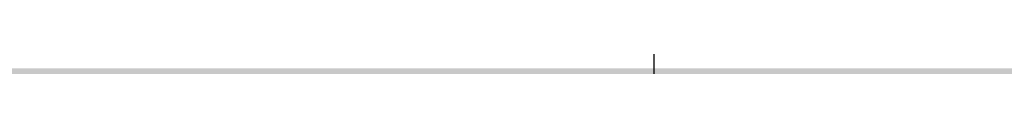
# Model space of a CAD drawing. Units: inches. Extents: x 2083 to 3317, y 1141 to 2115.
# Tile 61 of 256: x 2237.106 to 2238.294, y 1477.764 to 1477.769. Entities that reach past the tile are written whole.
import ezdxf

# ---------------------------------------------------------------- set-up
doc = ezdxf.new("R2010")
doc.units = ezdxf.units.IN
doc.layers.add('A-ANNO-DIMS', color=2, linetype='Continuous', lineweight=18)
doc.layers.add('A-WALL-PATT', color=251, linetype='Continuous', lineweight=13, true_color=0x636466)
doc.styles.get("Standard").update_dxf_attribs({"font": 'arial.ttf'})
doc.dimstyles.new('ISO-25', dxfattribs={"dimtxt": 12, "dimasz": 12, "dimexe": 1.25, "dimexo": 0.625, "dimtad": 1, "dimlunit": 3, "dimtxsty": 'Standard', "dimcen": 2.5, "dimadec": 0, "dimazin": 0, "dimtfac": 1, "dimtmove": 0, "dimatfit": 3, "dimfxl": 1, "dimarcsym": 0})

# ---------------------------------------------------------------- blocks, each defined once
blk = doc.blocks.new('*D30')
at = {"layer": 'A-ANNO-DIMS', "color": 0, "lineweight": -2, "transparency": 16777216}
for p, q in [((2240.0179, 1445.2738), (2240.0179, 1448.0455)), ((2254.3293, 1445.2738), (2254.3293, 1448.0455)), ((2228.0179, 1446.7955), (2216.0179, 1446.7955)), ((2240.0179, 1446.7955), (2254.3293, 1446.7955)), ((2266.3293, 1446.7955), (2413.7649, 1446.7955))]:
    blk.add_line(p, q, dxfattribs=at)
at = {"layer": 'A-ANNO-DIMS', "color": 0, "transparency": 16777216}
for points in [[(2228.0179, 1448.7955), (2228.0179, 1444.7955), (2240.0179, 1446.7955)], [(2266.3293, 1448.7955), (2266.3293, 1444.7955), (2254.3293, 1446.7955)]]:
    blk.add_solid(points, dxfattribs=at)
at = {"layer": 'Defpoints', "color": 0, "transparency": 16777216}
for p in [(2254.3293, 1446.7955), (2240.0179, 1444.6488), (2254.3293, 1444.6488)]:
    blk.add_point(p, dxfattribs=at)
at = {"layer": 'A-ANNO-DIMS', "color": 0, "transparency": 16777216, "insert": (2346.0471, 1453.6252), "char_height": 12, "attachment_point": 5}
blk.add_mtext('WC 1\'-2 1/2" TYP.', dxfattribs=at)
blk = doc.blocks.new('*D31')
at = {"layer": 'A-ANNO-DIMS', "color": 0, "lineweight": -2, "transparency": 16777216}
for p, q in [((2237.8711, 1456.6488), (2237.8711, 1541.9152)), ((2239.3929, 1444.6488), (2236.6211, 1444.6488)), ((2237.8711, 1431.5475), (2237.8711, 1444.6488)), ((2239.3929, 1431.5475), (2236.6211, 1431.5475)), ((2237.8711, 1419.5475), (2237.8711, 1407.5475))]:
    blk.add_line(p, q, dxfattribs=at)
at = {"layer": 'A-ANNO-DIMS', "color": 0, "transparency": 16777216}
for points in [[(2235.8711, 1456.6488), (2239.8711, 1456.6488), (2237.8711, 1444.6488)], [(2235.8711, 1419.5475), (2239.8711, 1419.5475), (2237.8711, 1431.5475)]]:
    blk.add_solid(points, dxfattribs=at)
at = {"layer": 'Defpoints', "color": 0, "transparency": 16777216}
for p in [(2237.8711, 1444.6488), (2240.0179, 1444.6488), (2240.0179, 1431.5475)]:
    blk.add_point(p, dxfattribs=at)
at = {"layer": 'A-ANNO-DIMS', "color": 0, "transparency": 16777216, "insert": (2231.2175, 1505.282), "char_height": 12, "attachment_point": 5, "rotation": 90}
blk.add_mtext('1\'-1" TYP.', dxfattribs=at)
blk = doc.blocks.new('*D45')
at = {"layer": 'A-ANNO-DIMS', "color": 0, "lineweight": -2, "transparency": 16777216}
for p, q in [((2235.9598, 1478.3864), (2235.9598, 1531.3614)), ((2418.9598, 1478.3864), (2418.9598, 1531.3614)), ((2247.9598, 1530.1114), (2406.9598, 1530.1114))]:
    blk.add_line(p, q, dxfattribs=at)
at = {"layer": 'A-ANNO-DIMS', "color": 0, "transparency": 16777216}
for points in [[(2247.9598, 1532.1114), (2247.9598, 1528.1114), (2235.9598, 1530.1114)], [(2406.9598, 1532.1114), (2406.9598, 1528.1114), (2418.9598, 1530.1114)]]:
    blk.add_solid(points, dxfattribs=at)
at = {"layer": 'Defpoints', "color": 0, "transparency": 16777216}
for p in [(2418.9598, 1530.1114), (2235.9598, 1477.7614), (2418.9598, 1477.7614)]:
    blk.add_point(p, dxfattribs=at)
at = {"layer": 'A-ANNO-DIMS', "color": 0, "transparency": 16777216, "insert": (2327.4598, 1536.8673), "char_height": 12, "attachment_point": 5}
blk.add_mtext('15\'-3"', dxfattribs=at)
blk = doc.blocks.new('*D62')
at = {"layer": 'A-ANNO-DIMS', "color": 0, "lineweight": -2, "transparency": 16777216}
for p, q in [((2235.9598, 1469.3864), (2235.9598, 1522.3614)), ((2379.9598, 1469.3864), (2379.9598, 1522.3614)), ((2247.9598, 1521.1114), (2367.9598, 1521.1114))]:
    blk.add_line(p, q, dxfattribs=at)
at = {"layer": 'A-ANNO-DIMS', "color": 0, "transparency": 16777216}
for points in [[(2247.9598, 1523.1114), (2247.9598, 1519.1114), (2235.9598, 1521.1114)], [(2367.9598, 1523.1114), (2367.9598, 1519.1114), (2379.9598, 1521.1114)]]:
    blk.add_solid(points, dxfattribs=at)
at = {"layer": 'Defpoints', "color": 0, "transparency": 16777216}
for p in [(2379.9598, 1521.1114), (2235.9598, 1468.7614), (2379.9598, 1468.7614)]:
    blk.add_point(p, dxfattribs=at)
at = {"layer": 'A-ANNO-DIMS', "color": 0, "transparency": 16777216, "insert": (2307.9598, 1527.8632), "char_height": 12, "attachment_point": 5}
blk.add_mtext('12\'-0"', dxfattribs=at)

msp = doc.modelspace()

# ---------------------------------------------------------------- hatches: boundary and pattern name
at = {"layer": 'A-WALL-PATT'}
h = msp.add_hatch(color=256, dxfattribs=at)
h.dxf.hatch_style = 1
h.paths.add_polyline_path([(3126.9598, 2020.7614), (2748.9598, 2020.7614), (2604.9598, 2020.7614), (2226.9598, 2020.7614), (2226.9598, 1702.7614), (2466.9598, 1702.7614), (2466.9598, 1582.7614), (2418.9598, 1582.7614), (2418.9598, 1477.7614), (2226.9598, 1477.7614), (2226.9598, 1263.2614), (2544.9598, 1263.2614), (2544.9598, 1411.7614), (2604.9598, 1411.7614), (2685.9598, 1411.7614), (2685.9598, 1420.7614), (2604.9598, 1420.7614), (2604.9598, 1573.7614), (2604.9598, 1702.7614), (2604.9598, 2011.7614), (2748.9598, 2011.7614), (2748.9598, 1702.7614), (2862.9598, 1702.7614), (2862.9598, 1621.7614), (2871.9598, 1621.7614), (2871.9598, 1702.7614), (2883.9598, 1702.7614), (2883.9598, 1706.9395, -0.026459), (2883.9598, 1711.7614), (2757.9598, 1711.7614), (2757.9598, 1807.7614), (2787.9598, 1807.7614), (2787.9598, 1812.2614), (2757.9598, 1812.2614), (2757.9598, 2011.7614), (2877.9598, 2011.7614), (2877.9598, 1812.2614), (2847.9598, 1812.2614), (2847.9598, 1807.7614), (2889.8357, 1807.7614), (2889.8357, 1812.2614), (2882.4598, 1812.2614), (2882.4598, 2011.7614), (3117.9598, 2011.7614), (3117.9598, 1812.2614), (2937.8357, 1812.2614), (2937.8357, 1807.7614), (2995.7098, 1807.7614), (2995.7098, 1796.1177), (3000.2098, 1796.1177), (3000.2098, 1807.7614), (3117.9598, 1807.7614), (3117.9598, 1711.7614), (3000.2098, 1711.7614), (3000.2098, 1760.1177), (2998.5727, 1760.1177, -0.020711), (2995.7098, 1760.1177), (2995.7098, 1711.7614), (2931.9598, 1711.7614), (2931.9598, 1702.7614), (3126.9598, 1702.7614)])
h.paths.add_polyline_path([(2471.4598, 2011.7614), (2471.4598, 1810.0114), (2462.7169, 1810.0114), (2462.7169, 1805.5114), (2505.9598, 1805.5114), (2505.9598, 1810.0114), (2475.9598, 1810.0114), (2475.9598, 2011.7614), (2595.9598, 2011.7614), (2595.9598, 1810.0114), (2565.9598, 1810.0114), (2565.9598, 1805.5114), (2595.9598, 1805.5114), (2595.9598, 1711.7614), (2235.9598, 1711.7614), (2235.9598, 1805.5114), (2353.7098, 1805.5114), (2353.7098, 1796.0542), (2358.2098, 1796.0542), (2358.2098, 1805.5114), (2414.7169, 1805.5114), (2414.7169, 1810.0114), (2235.9598, 1810.0114), (2235.9598, 2011.7614)], flags=16)
h.paths.add_polyline_path([(2270.2047, 1994.61), (2270.2047, 1970.61), (2246.2047, 1970.61), (2246.2047, 1994.61)], flags=0)
edge = h.paths.add_edge_path(flags=0)
edge.add_ellipse((2332.0274, 1899.7982), major_axis=(-3.043, 3.043), ratio=0.168252, start_angle=-161.3322, end_angle=-156.3071, ccw=False)
edge.add_ellipse((2333.082, 1898.7435), major_axis=(-1.0546, 1.0546), ratio=0.453532, start_angle=-123.371, end_angle=-94.1591)
edge = h.paths.add_edge_path(flags=0)
edge.add_ellipse((2332.0274, 1968.8763), major_axis=(3.043, 3.043), ratio=0.168252, start_angle=18.6678, end_angle=23.6929)
edge.add_spline(control_points=[(2332.9256, 1970.6911), (2332.2268, 1970.3361), (2330.8937, 1969.6589), (2328.4131, 1970.9321), (2327.2039, 1967.7487), (2324.7096, 1969.9556), (2322.5328, 1967.0124), (2320.0128, 1971.2958), (2317.6803, 1968.1578), (2316.0405, 1967.102), (2315.4269, 1966.8096)], knot_values=[0, 0, 0, 0, 2.267059, 4.324559, 6.685584, 8.878641, 11.121502, 14.300359, 17.755284, 19.732645, 19.732645, 19.732645, 19.732645], degree=3, periodic=0)
edge.add_ellipse((2332.0274, 1968.8763), major_axis=(3.043, 3.043), ratio=0.168252, start_angle=18.6678, end_angle=23.6929, ccw=False)
edge.add_ellipse((2333.082, 1969.9309), major_axis=(1.0546, 1.0546), ratio=0.453532, start_angle=56.629, end_angle=85.8409, ccw=False)
edge = h.paths.add_edge_path(flags=0)
edge.add_spline(control_points=[(2296.4283, 1967.9879), (2293.6278, 1965.3363), (2287.7036, 1959.7271), (2299.7439, 1949.9957), (2294.5326, 1935.6685), (2290.5732, 1920.6035), (2293.3941, 1909.9737), (2296.1854, 1904.9665)], knot_values=[0.099185, 0.099185, 0.099185, 0.099185, 0.345301, 0.619822, 0.982653, 1.386093, 1.810555, 1.810555, 1.810555, 1.810555], degree=3, periodic=0)
edge.add_spline(control_points=[(2296.1854, 1904.9665), (2297.3836, 1902.6193), (2298.001, 1901.9493), (2298.553, 1901.4682)], knot_values=[0.006246, 0.006246, 0.006246, 0.006246, 0.055476, 0.055476, 0.055476, 0.055476], degree=3, periodic=0)
edge.add_spline(control_points=[(2298.553, 1901.4682), (2297.2586, 1900.9232), (2295.2253, 1900.2321), (2293.0602, 1900.6142), (2292.1014, 1900.7884), (2292.0896, 1900.7906)], knot_values=[0.312835, 0.312835, 0.312835, 0.312835, 0.40178, 0.474987, 0.475903, 0.475903, 0.475903, 0.475903], degree=3, periodic=0)
edge.add_arc((2292.7936, 1904.6641), 3.937, 215.4209, 259.6982, ccw=False)
edge.add_spline(control_points=[(2289.5853, 1902.3823), (2289.4767, 1902.5351), (2289.3685, 1902.688), (2289.2609, 1902.8412)], knot_values=[0.102872, 0.102872, 0.102872, 0.102872, 0.116896, 0.116896, 0.116896, 0.116896], degree=3, periodic=0)
edge.add_spline(control_points=[(2289.2609, 1902.8412), (2288.6866, 1902.5502), (2287.64, 1902.0199), (2285.8813, 1901.874), (2283.853, 1901.5044), (2281.72, 1899.7105), (2278.467, 1899.4929), (2276.1571, 1901.8832), (2272.259, 1899.8041), (2267.7776, 1901.8432), (2262.2439, 1900.184), (2257.4149, 1901.7821), (2254.3184, 1900.7261), (2253.1783, 1900.3373)], knot_values=[0, 0, 0, 0, 1.907977, 3.477176, 5.261074, 7.972851, 11.680248, 13.717921, 16.939592, 22.789562, 27.502503, 33.595215, 37.145618, 37.145618, 37.145618, 37.145618], degree=3, periodic=0)
edge.add_line((2253.1783, 1900.3373), (2250.2442, 1902.8412))
edge.add_line((2250.2442, 1902.8412), (2250.2442, 1965.8333))
edge.add_line((2250.2442, 1965.8333), (2253.1783, 1968.3371))
edge.add_spline(control_points=[(2253.1783, 1968.3371), (2254.3184, 1967.9483), (2257.4149, 1966.8924), (2262.2439, 1968.4904), (2267.7776, 1966.8313), (2271.5267, 1968.5372), (2273.8759, 1967.8283), (2274.2067, 1967.7276)], knot_values=[0, 0, 0, 0, 0.09018, 0.244935, 0.364644, 0.513233, 0.537855, 0.537855, 0.537855, 0.537855], degree=3, periodic=0)
edge.add_arc((2274.3529, 1963.7933), 3.937, 72.0511, 92.1279, ccw=False)
edge.add_arc((2281.2969, 1985.23), 18.5963, 252.05113, 288.56572)
edge.add_arc((2292.3167, 1956.0289), 12.6461, 71.02679, 113.77822, ccw=False)
edge = h.paths.add_edge_path(flags=0)
edge.add_spline(control_points=[(2274.8994, 1951.8562), (2275.0662, 1951.6166), (2275.2327, 1951.3766), (2275.398, 1951.1359)], knot_values=[1.409916, 1.409916, 1.409916, 1.409916, 1.43159, 1.43159, 1.43159, 1.43159], degree=3, periodic=0)
edge.add_spline(control_points=[(2275.398, 1951.1359), (2275.7921, 1950.5619), (2276.1792, 1949.9838), (2276.5455, 1949.3971)], knot_values=[1.358238, 1.358238, 1.358238, 1.358238, 1.409916, 1.409916, 1.409916, 1.409916], degree=3, periodic=0)
edge.add_line((2276.5455, 1949.3971), (2277.4373, 1947.8622))
edge.add_spline(control_points=[(2277.4373, 1947.8622), (2276.3038, 1945.6731), (2274.6397, 1942.4269), (2274.6316, 1938.0939), (2272.7991, 1930.8515), (2274.3564, 1943.897), (2275.9477, 1947.9234), (2276.5455, 1949.3971)], knot_values=[0.005632, 0.005632, 0.005632, 0.005632, 0.186014, 0.266002, 0.357087, 0.59639, 0.739732, 0.739732, 0.739732, 0.739732], degree=3, periodic=0)
edge.add_spline(control_points=[(2276.5455, 1949.3971), (2276.1792, 1949.9838), (2275.7921, 1950.5619), (2275.398, 1951.1359)], knot_values=[1.358238, 1.358238, 1.358238, 1.358238, 1.409916, 1.409916, 1.409916, 1.409916], degree=3, periodic=0)
edge.add_spline(control_points=[(2275.398, 1951.1359), (2274.9425, 1950.0805), (2274.2078, 1948.0253), (2273.9346, 1944.8515), (2272.4685, 1937.6275), (2273.4662, 1945.6965), (2274.7006, 1951.0595), (2274.8994, 1951.8562)], knot_values=[0.104364, 0.104364, 0.104364, 0.104364, 0.189636, 0.269624, 0.36071, 0.600013, 0.644622, 0.644622, 0.644622, 0.644622], degree=3, periodic=0)
h.paths.add_polyline_path([(2269.1675, 1963.1276, -0.357527), (2268.1706, 1960.9764, -0.092561), (2268.1706, 1939.4363, -0.357527), (2269.1675, 1937.2851, -0.357527), (2267.0163, 1938.282, -0.164785), (2254.6856, 1938.282, -0.357527), (2252.5344, 1937.2851, -0.357527), (2253.5313, 1939.4363, -0.092561), (2253.5313, 1960.9764, -0.357527), (2252.5344, 1963.1276, -0.357527), (2254.6856, 1962.1307, -0.164785), (2267.0163, 1962.1307, -0.357527)], flags=0)
h.paths.add_polyline_path([(2248.8741, 1967.8018), (2248.8741, 1957.0277), (2249.4578, 1957.0277), (2249.4578, 1911.6468), (2248.8741, 1911.6468), (2248.8741, 1900.8727), (2246.5119, 1900.8727, 0.197327), (2244.1497, 1902.4569), (2244.1497, 1966.2176, 0.197327), (2246.5119, 1967.8018)], flags=0)
h.paths.add_polyline_path([(2269.1675, 1931.3893, -0.357527), (2268.1706, 1929.2381, -0.092561), (2268.1706, 1907.6981, -0.357527), (2269.1675, 1905.5469, -0.357527), (2267.0163, 1906.5438, -0.164785), (2254.6856, 1906.5438, -0.357527), (2252.5344, 1905.5469, -0.357527), (2253.5313, 1907.6981, -0.092561), (2253.5313, 1929.2381, -0.357527), (2252.5344, 1931.3893, -0.357527), (2254.6856, 1930.3925, -0.164785), (2267.0163, 1930.3925, -0.357527)], flags=0)
edge = h.paths.add_edge_path(flags=0)
edge.add_spline(control_points=[(2276.1969, 1906.7237), (2276.1681, 1909.0289), (2276.114, 1913.3719), (2270.5984, 1924.925), (2273.9052, 1919.0128), (2275.9217, 1916.2621), (2275.4746, 1912.4021), (2277.2579, 1910.3806), (2276.696, 1908.225), (2276.6462, 1906.813), (2276.6178, 1906.0084)], knot_values=[0, 0, 0, 0, 8.61026, 16.221274, 18.843057, 23.804898, 27.440828, 29.356102, 31.203478, 33.650687, 33.650687, 33.650687, 33.650687], degree=3, periodic=0)
edge.add_spline(control_points=[(2276.6178, 1906.0084), (2276.6233, 1905.6241), (2276.4977, 1904.6287), (2275.4418, 1903.8547), (2274.9373, 1903.0804), (2274.8591, 1902.8412)], knot_values=[0.156488, 0.156488, 0.156488, 0.156488, 0.184398, 0.231376, 0.250598, 0.250598, 0.250598, 0.250598], degree=3, periodic=0)
edge.add_line((2274.8591, 1902.8412), (2276.506, 1902.8412))
edge.add_spline(control_points=[(2276.506, 1902.8412), (2276.7883, 1903.0849), (2277.6651, 1904.1252), (2278.2495, 1904.3407), (2277.6539, 1908.5274), (2278.1557, 1906.2278), (2278.1005, 1905.2859), (2278.8467, 1904.069), (2277.8568, 1903.4149), (2277.8742, 1902.991), (2277.9036, 1902.8412)], knot_values=[0.059574, 0.059574, 0.059574, 0.059574, 0.080753, 0.103741, 0.16972, 0.176036, 0.207137, 0.240474, 0.262341, 0.27366, 0.27366, 0.27366, 0.27366], degree=3, periodic=0)
edge.add_line((2277.9036, 1902.8412), (2280.0298, 1902.8412))
edge.add_spline(control_points=[(2280.0298, 1902.8412), (2279.8882, 1903.0884), (2279.4993, 1903.9816), (2280.1523, 1905.9393), (2278.1036, 1909.6578), (2279.7624, 1907.1853), (2280.3279, 1904.8749), (2280.4851, 1903.4896), (2281.4633, 1903.2494), (2281.7583, 1902.9365), (2281.834, 1902.8412)], knot_values=[0.013856, 0.013856, 0.013856, 0.013856, 0.034874, 0.088867, 0.107879, 0.126738, 0.158714, 0.193757, 0.217487, 0.226722, 0.226722, 0.226722, 0.226722], degree=3, periodic=0)
edge.add_spline(control_points=[(2281.834, 1902.8412), (2281.7875, 1902.8267), (2281.647, 1902.783), (2281.3955, 1902.8595), (2281.0881, 1902.9852), (2280.7207, 1903.0609), (2280.3335, 1903.0257), (2280.1248, 1902.8989), (2280.0298, 1902.8412)], knot_values=[0, 0, 0, 0, 0.14413, 0.435517, 0.749276, 1.153046, 1.548371, 1.878348, 1.878348, 1.878348, 1.878348], degree=3, periodic=0)
edge.add_line((2280.0298, 1902.8412), (2277.9036, 1902.8412))
edge.add_spline(control_points=[(2277.9036, 1902.8412), (2277.8929, 1902.7959), (2277.8654, 1902.6796), (2277.6075, 1902.6875), (2277.2741, 1902.8007), (2276.8379, 1902.6198), (2276.5838, 1902.7893), (2276.506, 1902.8412)], knot_values=[0, 0, 0, 0, 0.127189, 0.326199, 0.628009, 1.24357, 1.515331, 1.515331, 1.515331, 1.515331], degree=3, periodic=0)
edge.add_line((2276.506, 1902.8412), (2274.8591, 1902.8412))
edge.add_spline(control_points=[(2274.8591, 1902.8412), (2274.8144, 1902.8986), (2274.7251, 1903.0134), (2274.4935, 1903.119), (2274.2443, 1902.9605), (2273.9371, 1903.1849), (2273.614, 1902.9831), (2273.4083, 1902.883), (2273.3223, 1902.8412)], knot_values=[0, 0, 0, 0, 0.21843, 0.436957, 0.687977, 0.990379, 1.398396, 1.69185, 1.69185, 1.69185, 1.69185], degree=3, periodic=0)
edge.add_spline(control_points=[(2273.3223, 1902.8412), (2273.6167, 1903.4457), (2274.274, 1904.5383), (2276.0272, 1904.5737), (2276.207, 1906.5836), (2276.1969, 1906.7237)], knot_values=[0.012227, 0.012227, 0.012227, 0.012227, 0.059472, 0.106218, 0.134458, 0.134458, 0.134458, 0.134458], degree=3, periodic=0)
h.paths.add_polyline_path([(2270.7761, 1897.7898), (2270.7761, 1873.7898), (2246.7761, 1873.7898), (2246.7761, 1897.7898)], flags=0)
h.paths.add_polyline_path([(2353.7098, 1760.0051), (2353.7098, 1760.0542), (2358.2098, 1760.0542, -0.033729)], flags=0)
h.paths.add_polyline_path([(2321.8191, 1737.5292), (2341.9953, 1737.5292, -0.414214), (2343.2033, 1736.3212), (2343.2033, 1721.0206, -0.414214), (2341.9953, 1719.8127), (2321.8191, 1719.8127, -0.414214), (2320.6112, 1721.0206), (2320.6112, 1736.3212, -0.414214)], flags=0)
h.paths.add_polyline_path([(2324.235, 1736.3212), (2339.5794, 1736.3212, -0.414214), (2341.9953, 1733.9053), (2341.9953, 1725.4497, -0.414214), (2339.5794, 1723.0338), (2333.6806, 1723.0338), (2333.8453, 1722.0455, -0.870646), (2335.4254, 1721.8259, -0.767327), (2333.9227, 1721.4232), (2331.291, 1721.4232, -0.767327), (2329.7883, 1721.8259, -0.870646), (2331.3684, 1722.0455), (2331.5331, 1723.0338), (2324.235, 1723.0338, -0.414214), (2321.8191, 1725.4497), (2321.8191, 1733.9053, -0.414214)], flags=0)
h.paths.add_polyline_path([(2570.4838, 1928.6154), (2589.6838, 1928.6154), (2590.1688, 1928.6154), (2590.1688, 1904.9934), (2570.4838, 1904.9934)], flags=0)
h.paths.add_polyline_path([(2574.4473, 1927.2638, -1), (2572.8288, 1927.2638, -1)], flags=0)
h.paths.add_polyline_path([(2573.0899, 1926.9409), (2573.925, 1927.776), (2574.1477, 1927.5533), (2573.3126, 1926.7182)], flags=0)
h.paths.add_polyline_path([(2578.7791, 1919.7296, -1), (2571.5917, 1919.7296, -1)], flags=0)
h.paths.add_polyline_path([(2578.3854, 1919.7296, -1), (2571.9854, 1919.7296, -1)], flags=0)
h.paths.add_polyline_path([(2331.5958, 1729.4762, -1), (2333.618, 1729.4762, -1)], flags=0)
h.paths.add_polyline_path([(2578.0342, 1927.2638, -1), (2576.4157, 1927.2638, -1)], flags=0)
h.paths.add_polyline_path([(2576.6889, 1927.5311), (2576.9116, 1927.7538), (2577.7467, 1926.9186), (2577.524, 1926.6959)], flags=0)
h.paths.add_polyline_path([(2578.1391, 1909.8595, -1), (2572.2317, 1909.8595, -1)], flags=0)
h.paths.add_polyline_path([(2577.7454, 1909.8595, -1), (2572.6254, 1909.8595, -1)], flags=0)
h.paths.add_polyline_path([(2583.7977, 1927.2638, -1), (2582.1792, 1927.2638, -1)], flags=0)
h.paths.add_polyline_path([(2582.7186, 1927.7538), (2583.5538, 1926.9186), (2583.3311, 1926.6959), (2582.4959, 1927.5311)], flags=0)
h.paths.add_polyline_path([(2582.4959, 1927.5311), (2582.7186, 1927.7538), (2583.5538, 1926.9186), (2583.3311, 1926.6959)], flags=0)
h.paths.add_polyline_path([(2587.7391, 1920.5296, -1), (2581.8317, 1920.5296, -1)], flags=0)
h.paths.add_polyline_path([(2587.3454, 1920.5296, -1), (2582.2254, 1920.5296, -1)], flags=0)
h.paths.add_polyline_path([(2587.3846, 1927.2638, -1), (2585.7661, 1927.2638, -1)], flags=0)
h.paths.add_polyline_path([(2586.082, 1926.9802), (2586.9172, 1927.8154), (2587.1399, 1927.5927), (2586.3047, 1926.7575)], flags=0)
h.paths.add_polyline_path([(2588.3791, 1910.6595, -1), (2581.1917, 1910.6595, -1)], flags=0)
h.paths.add_polyline_path([(2587.9854, 1910.6595, -1), (2581.5854, 1910.6595, -1)], flags=0)
h.paths.add_polyline_path([(2417.1677, 1729.4779), (2437.3439, 1729.4779, -0.414214), (2438.5519, 1728.2699), (2438.5519, 1712.9693, -0.414214), (2437.3439, 1711.7614), (2417.1677, 1711.7614, -0.414214), (2415.9598, 1712.9693), (2415.9598, 1728.2699, -0.414214)], flags=0)
h.paths.add_polyline_path([(2419.5836, 1728.2699), (2434.928, 1728.2699, -0.414214), (2437.3439, 1725.8541), (2437.3439, 1717.3984, -0.414214), (2434.928, 1714.9825), (2429.0292, 1714.9825), (2429.1939, 1713.9942, -0.870646), (2430.774, 1713.7746, -0.767327), (2429.2713, 1713.372), (2426.6396, 1713.372, -0.767327), (2425.1369, 1713.7746, -0.870646), (2426.717, 1713.9942), (2426.8817, 1714.9825), (2419.5836, 1714.9825, -0.414214), (2417.1677, 1717.3984), (2417.1677, 1725.8541, -0.414214)], flags=0)
h.paths.add_polyline_path([(2419.5836, 1728.2699), (2434.928, 1728.2699, -0.414214), (2437.3439, 1725.8541), (2437.3439, 1717.3984, -0.414214), (2434.928, 1714.9825), (2429.0292, 1714.9825), (2428.3581, 1719.009), (2427.5528, 1719.009), (2426.8817, 1714.9825), (2419.5836, 1714.9825, -0.414214), (2417.1677, 1717.3984), (2417.1677, 1725.8541, -0.414214)], flags=0)
h.paths.add_polyline_path([(2426.9444, 1721.4249, -1), (2428.9666, 1721.4249, -1)], flags=0)
h.paths.add_polyline_path([(2475.9598, 1702.7614), (2595.9598, 1702.7614), (2595.9598, 1582.7614), (2475.9598, 1582.7614)], flags=16)
h.paths.add_polyline_path([(2427.9598, 1573.7614), (2595.9598, 1573.7614), (2595.9598, 1468.7614), (2595.9598, 1420.7614), (2384.4598, 1420.7614), (2384.4598, 1468.7614), (2427.9598, 1468.7614)], flags=16)
h.paths.add_polyline_path([(2379.9598, 1468.7614), (2379.9598, 1420.7614), (2235.9598, 1420.7614), (2235.9598, 1468.7614)], flags=16)
h.paths.add_polyline_path([(2317.816, 1466.6958), (2337.9922, 1466.6958, -0.414214), (2339.2002, 1465.4878), (2339.2002, 1450.1872, -0.414214), (2337.9922, 1448.9792), (2317.816, 1448.9792, -0.414214), (2316.6081, 1450.1872), (2316.6081, 1465.4878, -0.414214)], flags=0)
h.paths.add_polyline_path([(2320.2319, 1465.4878), (2335.5763, 1465.4878, -0.414214), (2337.9922, 1463.0719), (2337.9922, 1454.6163, -0.414214), (2335.5763, 1452.2004), (2329.6775, 1452.2004), (2329.8422, 1451.212, -0.870646), (2331.4223, 1450.9925, -0.767327), (2329.9196, 1450.5898), (2327.2879, 1450.5898, -0.767327), (2325.7852, 1450.9925, -0.870646), (2327.3653, 1451.212), (2327.53, 1452.2004), (2320.2319, 1452.2004, -0.414214), (2317.816, 1454.6163), (2317.816, 1463.0719, -0.414214)], flags=0)
h.paths.add_polyline_path([(2320.2319, 1465.4878), (2335.5763, 1465.4878, -0.414214), (2337.9922, 1463.0719), (2337.9922, 1454.6163, -0.414214), (2335.5763, 1452.2004), (2329.6775, 1452.2004), (2329.0064, 1456.2269), (2328.2011, 1456.2269), (2327.53, 1452.2004), (2320.2319, 1452.2004, -0.414214), (2317.816, 1454.6163), (2317.816, 1463.0719, -0.414214)], flags=0)
h.paths.add_polyline_path([(2327.5926, 1458.6428, -1), (2329.6148, 1458.6428, -1)], flags=0)
h.paths.add_polyline_path([(2244.4117, 1433.3405), (2241.9209, 1433.3405, -0.414214), (2240.0179, 1435.2435), (2240.0179, 1440.9528, -0.414211), (2241.9209, 1442.8559), (2244.4117, 1442.8559, -1.976472)], flags=0)
h.paths.add_polyline_path([(2245.3569, 1434.3975, -0.414214), (2245.3569, 1441.7988, -2.144098)], flags=0)
h.paths.add_polyline_path([(2535.9598, 1416.2614), (2535.9598, 1272.2614), (2235.9598, 1272.2614), (2235.9598, 1416.2614)], flags=16)
h.paths.add_polyline_path([(2260.1196, 1384.2928), (2260.1196, 1362.0386), (2237.8654, 1362.0386), (2237.8654, 1384.2928)], flags=0)
edge = h.paths.add_edge_path(flags=0)
edge.add_line((2318.2518, 1362.0933), (2318.1458, 1362.001))
edge.add_ellipse((2317.4451, 1360.431), major_axis=(2.8216, 2.8216), ratio=0.168252, start_angle=18.6678, end_angle=20.9481, ccw=False)
edge.add_ellipse((2318.423, 1361.409), major_axis=(0.9779, 0.9779), ratio=0.453532, start_angle=56.629, end_angle=70.2262, ccw=False)
edge = h.paths.add_edge_path(flags=0)
edge.add_line((2319.1074, 1295.5711), (2319.015, 1295.6771))
edge.add_ellipse((2317.4451, 1296.3778), major_axis=(-2.8216, 2.8216), ratio=0.168252, start_angle=-161.3322, end_angle=-159.0519, ccw=False)
edge.add_ellipse((2318.423, 1295.3999), major_axis=(-0.9779, 0.9779), ratio=0.453532, start_angle=-123.371, end_angle=-109.7738)
edge = h.paths.add_edge_path(flags=0)
edge.add_spline(control_points=[(2284.2103, 1301.1702), (2284.5807, 1300.4447), (2284.8912, 1299.892), (2285.1596, 1299.461)], knot_values=[0.039066, 0.039066, 0.039066, 0.039066, 0.055476, 0.055476, 0.055476, 0.055476], degree=3, periodic=0)
edge.add_line((2285.1596, 1299.461), (2284.2103, 1301.1702))
edge = h.paths.add_edge_path(flags=0)
edge.add_line((2280.4125, 1297.298), (2283.37, 1297.0361))
edge.add_line((2283.37, 1297.0361), (2286.4057, 1297.9263))
edge.add_spline(control_points=[(2286.4057, 1297.9263), (2285.3055, 1297.4631), (2284.3448, 1297.1292), (2283.37, 1297.0361)], knot_values=[0.394369, 0.394369, 0.394369, 0.394369, 0.475903, 0.475903, 0.475903, 0.475903], degree=3, periodic=0)
edge.add_spline(control_points=[(2283.37, 1297.0361), (2283.2814, 1297.0277), (2282.3163, 1296.9573), (2281.3125, 1297.1345), (2280.4234, 1297.296), (2280.4125, 1297.298)], knot_values=[0.312835, 0.312835, 0.312835, 0.312835, 0.320246, 0.393453, 0.394369, 0.394369, 0.394369, 0.394369], degree=3, periodic=0)
edge = h.paths.add_edge_path(flags=0)
edge.add_line((2284.4356, 1359.6073), (2280.4463, 1355.328))
edge.add_line((2280.4463, 1355.328), (2279.58, 1351.0178))
edge.add_line((2279.58, 1351.0178), (2282.413, 1346.5804))
edge.add_spline(control_points=[(2282.413, 1346.5804), (2283.1533, 1345.5892), (2284.2529, 1344.0289), (2284.801, 1342.3872), (2284.9352, 1341.8055)], knot_values=[1.240098, 1.240098, 1.240098, 1.240098, 1.332892, 1.382712, 1.382712, 1.382712, 1.382712], degree=3, periodic=0)
edge.add_spline(control_points=[(2284.9352, 1341.8055), (2285.3191, 1340.1406), (2285.233, 1338.4092), (2284.9099, 1336.6541)], knot_values=[1.097484, 1.097484, 1.097484, 1.097484, 1.240098, 1.240098, 1.240098, 1.240098], degree=3, periodic=0)
edge.add_spline(control_points=[(2284.9099, 1336.6541), (2284.5868, 1334.899), (2284.0267, 1333.1203), (2283.4626, 1331.3606)], knot_values=[0.95487, 0.95487, 0.95487, 0.95487, 1.097484, 1.097484, 1.097484, 1.097484], degree=3, periodic=0)
edge.add_line((2283.4626, 1331.3606), (2281.8904, 1326.1534))
edge.add_line((2281.8904, 1326.1534), (2280.7563, 1321.0561))
edge.add_line((2280.7563, 1321.0561), (2280.2992, 1316.002))
edge.add_line((2280.2992, 1316.002), (2280.7159, 1310.9501))
edge.add_line((2280.7159, 1310.9501), (2282.0281, 1305.9721))
edge.add_line((2282.0281, 1305.9721), (2284.2103, 1301.1702))
edge.add_spline(control_points=[(2284.2103, 1301.1702), (2283.3407, 1302.7302), (2282.6119, 1304.3365), (2282.0281, 1305.9721)], knot_values=[0.099185, 0.099185, 0.099185, 0.099185, 0.241799, 0.241799, 0.241799, 0.241799], degree=3, periodic=0)
edge.add_spline(control_points=[(2282.0281, 1305.9721), (2281.4443, 1307.6078), (2281.0055, 1309.2728), (2280.7159, 1310.9501)], knot_values=[0.241799, 0.241799, 0.241799, 0.241799, 0.384413, 0.384413, 0.384413, 0.384413], degree=3, periodic=0)
edge.add_spline(control_points=[(2280.7159, 1310.9501), (2280.4332, 1312.5876), (2280.2894, 1314.277), (2280.2989, 1315.962), (2280.2992, 1316.002)], knot_values=[0.384413, 0.384413, 0.384413, 0.384413, 0.523647, 0.527028, 0.527028, 0.527028, 0.527028], degree=3, periodic=0)
edge.add_spline(control_points=[(2280.2992, 1316.002), (2280.3123, 1317.687), (2280.4779, 1319.3679), (2280.7563, 1321.0561)], knot_values=[0.527028, 0.527028, 0.527028, 0.527028, 0.669642, 0.669642, 0.669642, 0.669642], degree=3, periodic=0)
edge.add_spline(control_points=[(2280.7563, 1321.0561), (2281.0346, 1322.7443), (2281.4259, 1324.4396), (2281.8904, 1326.1534)], knot_values=[0.669642, 0.669642, 0.669642, 0.669642, 0.812256, 0.812256, 0.812256, 0.812256], degree=3, periodic=0)
edge.add_spline(control_points=[(2281.8904, 1326.1534), (2282.2644, 1327.5333), (2282.7879, 1329.2618), (2283.3528, 1331.0178), (2283.4626, 1331.3606)], knot_values=[0.812256, 0.812256, 0.812256, 0.812256, 0.927087, 0.95487, 0.95487, 0.95487, 0.95487], degree=3, periodic=0)
edge.add_line((2283.4626, 1331.3606), (2284.9099, 1336.6541))
edge.add_line((2284.9099, 1336.6541), (2284.9352, 1341.8055))
edge.add_line((2284.9352, 1341.8055), (2282.413, 1346.5804))
edge.add_spline(control_points=[(2282.413, 1346.5804), (2281.2751, 1348.1038), (2280.0784, 1349.5703), (2279.58, 1351.0178)], knot_values=[1.382712, 1.382712, 1.382712, 1.382712, 1.525326, 1.525326, 1.525326, 1.525326], degree=3, periodic=0)
edge.add_spline(control_points=[(2279.58, 1351.0178), (2279.4433, 1351.4147), (2279.1363, 1352.8569), (2279.7352, 1354.2904), (2280.4463, 1355.328)], knot_values=[1.525326, 1.525326, 1.525326, 1.525326, 1.564439, 1.667941, 1.667941, 1.667941, 1.667941], degree=3, periodic=0)
edge.add_spline(control_points=[(2280.4463, 1355.328), (2281.4261, 1356.7578), (2282.9308, 1358.1826), (2284.4356, 1359.6073)], knot_values=[1.667941, 1.667941, 1.667941, 1.667941, 1.810555, 1.810555, 1.810555, 1.810555], degree=3, periodic=0)
edge.add_arc((2280.6231, 1348.5182), 11.7262, 71.02679, 113.77822)
edge.add_arc((2270.4049, 1375.5952), 17.2436, 252.05113, 288.56572, ccw=False)
edge.add_arc((2263.966, 1355.7178), 3.6506, 72.0511, 92.1279)
edge.add_arc((2263.966, 1355.7178), 3.6506, 92.1279, 177.9851)
edge.add_spline(control_points=[(2260.3176, 1355.8462), (2260.2604, 1354.2207), (2260.5513, 1350.1865), (2262.9993, 1346.7663), (2264.4727, 1344.649)], knot_values=[1.43159, 1.43159, 1.43159, 1.43159, 1.564144, 1.770695, 1.770695, 1.770695, 1.770695], degree=3, periodic=0)
edge.add_line((2264.4727, 1344.649), (2264.9356, 1343.9825))
edge.add_spline(control_points=[(2263.801, 1340.2481), (2263.8432, 1340.5141), (2264.0672, 1341.7565), (2264.5127, 1343.0025), (2264.935, 1343.9811)], knot_values=[0.53657, 0.53657, 0.53657, 0.53657, 0.559349, 0.644622, 0.644622, 0.644622, 0.644622], degree=3, periodic=0)
edge.add_spline(control_points=[(2264.935, 1343.9811), (2265.1178, 1343.715), (2265.2989, 1343.4479), (2265.4768, 1343.1794)], knot_values=[1.384077, 1.384077, 1.384077, 1.384077, 1.409916, 1.409916, 1.409916, 1.409916], degree=3, periodic=0)
edge.add_spline(control_points=[(2265.4768, 1343.1794), (2265.6546, 1342.9108), (2265.8293, 1342.6408), (2265.9991, 1342.3688)], knot_values=[1.358238, 1.358238, 1.358238, 1.358238, 1.384077, 1.384077, 1.384077, 1.384077], degree=3, periodic=0)
edge.add_line((2265.9991, 1342.3688), (2266.826, 1340.9455))
edge.add_spline(control_points=[(2266.826, 1340.9455), (2268.8944, 1337.0897), (2271.3982, 1325.843), (2270.5162, 1310.5686), (2275.9194, 1301.8606), (2277.7895, 1299.1994)], knot_values=[0.116896, 0.116896, 0.116896, 0.116896, 0.472987, 1.050969, 1.313793, 1.313793, 1.313793, 1.313793], degree=3, periodic=0)
edge.add_spline(control_points=[(2277.7895, 1299.1994), (2277.8394, 1299.1285), (2277.8894, 1299.0575), (2277.9396, 1298.9866)], knot_values=[0.109884, 0.109884, 0.109884, 0.109884, 0.116896, 0.116896, 0.116896, 0.116896], degree=3, periodic=0)
edge.add_line((2277.9396, 1298.9866), (2277.7888, 1299.1991))
edge.add_spline(control_points=[(2277.7888, 1299.1991), (2277.2566, 1298.9294), (2276.2864, 1298.4379), (2275.0394, 1298.3344), (2274.3833, 1298.2389), (2274.2153, 1298.2093)], knot_values=[33.12187, 33.12187, 33.12187, 33.12187, 35.029056, 36.598255, 37.144827, 37.144827, 37.144827, 37.144827], degree=3, periodic=0)
edge.add_line((2274.2153, 1298.2093), (2273.0731, 1297.893))
edge.add_spline(control_points=[(2273.0731, 1297.893), (2272.3229, 1297.5798), (2271.0392, 1296.5105), (2269.2484, 1296.2261), (2268.4231, 1296.3747)], knot_values=[26.532584, 26.532584, 26.532584, 26.532584, 29.198919, 31.839101, 31.839101, 31.839101, 31.839101], degree=3, periodic=0)
edge.add_line((2268.4231, 1296.3747), (2263.8785, 1297.4575))
edge.add_spline(control_points=[(2263.8785, 1297.4575), (2263.5561, 1297.3594), (2261.8603, 1296.8387), (2260.2388, 1297.2824), (2258.9335, 1297.5165)], knot_values=[15.919551, 15.919551, 15.919551, 15.919551, 16.939592, 21.226067, 21.226067, 21.226067, 21.226067], degree=3, periodic=0)
edge.add_line((2258.9335, 1297.5165), (2254.0552, 1297.329))
edge.add_spline(control_points=[(2254.0552, 1297.329), (2253.7555, 1297.2958), (2252.1137, 1297.1652), (2250.4619, 1297.5442), (2249.1297, 1297.6679)], knot_values=[5.306517, 5.306517, 5.306517, 5.306517, 6.276435, 10.613034, 10.613034, 10.613034, 10.613034], degree=3, periodic=0)
edge.add_line((2249.1297, 1297.6679), (2244.3316, 1296.8778))
edge.add_line((2244.3316, 1296.8778), (2241.611, 1299.1994))
edge.add_line((2241.611, 1299.1994), (2241.611, 1357.6094))
edge.add_line((2241.611, 1357.6094), (2244.3316, 1359.9311))
edge.add_line((2244.3316, 1359.9311), (2252.7288, 1359.5427))
edge.add_spline(control_points=[(2252.7288, 1359.5427), (2252.8709, 1359.5464), (2253.3057, 1359.5482), (2253.7398, 1359.5143), (2254.0317, 1359.4824)], knot_values=[0.233291, 0.233291, 0.233291, 0.233291, 0.244935, 0.268927, 0.268927, 0.268927, 0.268927], degree=3, periodic=0)
edge.add_line((2254.0317, 1359.4824), (2259.5872, 1359.4164))
edge.add_spline(control_points=[(2259.5872, 1359.4164), (2260.6771, 1359.6285), (2262.0732, 1359.897), (2263.5237, 1359.4593), (2263.8304, 1359.366)], knot_values=[0.422516, 0.422516, 0.422516, 0.422516, 0.513233, 0.537855, 0.537855, 0.537855, 0.537855], degree=3, periodic=0)
edge.add_arc((2263.966, 1355.7178), 3.6506, 72.0511, 92.1279, ccw=False)
edge.add_arc((2270.4049, 1375.5952), 17.2436, 252.05113, 288.56572)
edge.add_arc((2280.6231, 1348.5182), 11.7262, 71.02679, 113.77822, ccw=False)
h.paths.add_polyline_path([(2240.3405, 1359.4347), (2240.3405, 1349.4444), (2240.8818, 1349.4444), (2240.8818, 1307.3645), (2240.3405, 1307.3645), (2240.3405, 1297.3741), (2238.1502, 1297.3741, 0.197327), (2235.9598, 1298.8431), (2235.9598, 1357.9657, 0.197327), (2238.1502, 1359.4347)], flags=0)
h.paths.add_polyline_path([(2259.1578, 1355.1005, -0.357527), (2258.2334, 1353.1058, -0.092561), (2258.2334, 1333.1326, -0.357527), (2259.1578, 1331.1379, -0.357527), (2257.1631, 1332.0622, -0.164785), (2245.7293, 1332.0622, -0.357527), (2243.7346, 1331.1379, -0.357527), (2244.6589, 1333.1326, -0.092561), (2244.6589, 1353.1058, -0.357527), (2243.7346, 1355.1005, -0.357527), (2245.7293, 1354.1761, -0.164785), (2257.1631, 1354.1761, -0.357527)], flags=0)
edge = h.paths.add_edge_path(flags=0)
edge.add_line((2265.9991, 1342.3688), (2266.826, 1340.9455))
edge.add_line((2266.826, 1340.9455), (2265.3076, 1337.8141))
edge.add_line((2265.3076, 1337.8141), (2264.3582, 1334.6529))
edge.add_line((2264.3582, 1334.6529), (2264.262, 1333.7997))
edge.add_spline(control_points=[(2264.262, 1333.7997), (2264.2084, 1333.1871), (2264.1621, 1332.3655), (2264.0071, 1331.4139), (2263.969, 1331.2018)], knot_values=[0.464444, 0.464444, 0.464444, 0.464444, 0.516691, 0.531608, 0.531608, 0.531608, 0.531608], degree=3, periodic=0)
edge.add_spline(control_points=[(2263.969, 1331.2018), (2263.7745, 1330.1189), (2263.4244, 1328.7908), (2263.2574, 1328.5307), (2263.234, 1328.5146)], knot_values=[0.372682, 0.372682, 0.372682, 0.372682, 0.44885, 0.464444, 0.464444, 0.464444, 0.464444], degree=3, periodic=0)
edge.add_spline(control_points=[(2263.234, 1328.5146), (2263.0964, 1328.4202), (2263.1312, 1329.3015), (2263.275, 1330.6157)], knot_values=[0.280919, 0.280919, 0.280919, 0.280919, 0.372682, 0.372682, 0.372682, 0.372682], degree=3, periodic=0)
edge.add_spline(control_points=[(2263.275, 1330.6157), (2263.4187, 1331.93), (2263.6715, 1333.6773), (2263.9699, 1335.315)], knot_values=[0.189157, 0.189157, 0.189157, 0.189157, 0.280919, 0.280919, 0.280919, 0.280919], degree=3, periodic=0)
edge.add_spline(control_points=[(2263.9699, 1335.315), (2264.1005, 1336.0322), (2264.4188, 1337.6219), (2264.7548, 1338.8644), (2264.9474, 1339.4911)], knot_values=[0.097394, 0.097394, 0.097394, 0.097394, 0.137578, 0.189157, 0.189157, 0.189157, 0.189157], degree=3, periodic=0)
edge.add_spline(control_points=[(2264.9474, 1339.4911), (2265.29, 1340.6061), (2265.6442, 1341.494), (2265.9991, 1342.3688)], knot_values=[0.005632, 0.005632, 0.005632, 0.005632, 0.097394, 0.097394, 0.097394, 0.097394], degree=3, periodic=0)
h.paths.add_polyline_path([(2259.1578, 1325.671, -0.357527), (2258.2334, 1323.6763, -0.092561), (2258.2334, 1303.7031, -0.357527), (2259.1578, 1301.7084, -0.357527), (2257.1631, 1302.6327, -0.164785), (2245.7293, 1302.6327, -0.357527), (2243.7346, 1301.7084, -0.357527), (2244.6589, 1303.7031, -0.092561), (2244.6589, 1323.6763, -0.357527), (2243.7346, 1325.671, -0.357527), (2245.7293, 1324.7466, -0.164785), (2257.1631, 1324.7466, -0.357527)], flags=0)
edge = h.paths.add_edge_path(flags=0)
edge.add_spline(control_points=[(2261.7089, 1317.3114), (2261.6795, 1317.4176), (2261.7619, 1317.3885), (2262.4907, 1316.0899), (2262.9622, 1315.3009)], knot_values=[14.955861, 14.955861, 14.955861, 14.955861, 16.221274, 18.694826, 18.694826, 18.694826, 18.694826], degree=3, periodic=0)
edge.add_spline(control_points=[(2262.9622, 1315.3009), (2262.9904, 1315.2536), (2263.7021, 1314.0674), (2264.349, 1313.1272), (2264.7301, 1312.1642)], knot_values=[18.694826, 18.694826, 18.694826, 18.694826, 18.843057, 22.433791, 22.433791, 22.433791, 22.433791], degree=3, periodic=0)
edge.add_spline(control_points=[(2264.7301, 1312.1642), (2264.8756, 1311.7964), (2265.1769, 1310.7698), (2265.1431, 1309.5593), (2265.2477, 1308.8242)], knot_values=[22.433791, 22.433791, 22.433791, 22.433791, 23.804898, 26.172756, 26.172756, 26.172756, 26.172756], degree=3, periodic=0)
edge.add_line((2265.2477, 1308.8242), (2265.8508, 1307.1719))
edge.add_spline(control_points=[(2265.8508, 1307.1719), (2266.065, 1306.8217), (2266.3844, 1306.3322), (2266.4244, 1305.7805), (2266.4204, 1305.6112)], knot_values=[28.062562, 28.062562, 28.062562, 28.062562, 29.356102, 29.911721, 29.911721, 29.911721, 29.911721], degree=3, periodic=0)
edge.add_spline(control_points=[(2266.4204, 1305.6112), (2266.4161, 1305.4326), (2266.394, 1305.25), (2266.3648, 1305.0659)], knot_values=[29.911721, 29.911721, 29.911721, 29.911721, 30.497837, 30.497837, 30.497837, 30.497837], degree=3, periodic=0)
edge.add_line((2266.3648, 1305.0659), (2266.0662, 1302.1363))
edge.add_spline(control_points=[(2266.0662, 1302.1363), (2266.0712, 1301.78), (2265.9981, 1301.2), (2265.6633, 1300.759), (2265.5089, 1300.5859)], knot_values=[0.156488, 0.156488, 0.156488, 0.156488, 0.184398, 0.203543, 0.203543, 0.203543, 0.203543], degree=3, periodic=0)
edge.add_line((2265.5089, 1300.5859), (2264.4353, 1299.1994))
edge.add_line((2264.4353, 1299.1994), (2265.9624, 1299.1994))
edge.add_line((2265.9624, 1299.1994), (2267.336, 1301.1753))
edge.add_line((2267.336, 1301.1753), (2267.3117, 1301.9862))
edge.add_spline(control_points=[(2267.3117, 1301.9862), (2267.2611, 1302.8624), (2267.1602, 1303.7371), (2267.2715, 1303.3259)], knot_values=[0.126229, 0.126229, 0.126229, 0.126229, 0.166617, 0.166617, 0.166617, 0.166617], degree=3, periodic=0)
edge.add_spline(control_points=[(2267.2715, 1303.3259), (2267.28, 1303.2943), (2267.3098, 1303.1754), (2267.3735, 1302.8836), (2267.4061, 1302.6828), (2267.4179, 1302.601)], knot_values=[0.166617, 0.166617, 0.166617, 0.166617, 0.16972, 0.176036, 0.180765, 0.180765, 0.180765, 0.180765], degree=3, periodic=0)
edge.add_spline(control_points=[(2267.7439, 1300.9875), (2267.6876, 1301.1509), (2267.4805, 1301.6567), (2267.4838, 1302.1448), (2267.4179, 1302.601)], knot_values=[0.180765, 0.180765, 0.180765, 0.180765, 0.193767, 0.220139, 0.220139, 0.220139, 0.220139], degree=3, periodic=0)
edge.add_line((2267.4179, 1302.601), (2267.7439, 1300.9875))
edge.add_spline(control_points=[(2267.7439, 1300.9875), (2267.832, 1300.7319), (2267.932, 1300.3099), (2267.5548, 1299.9745), (2267.4294, 1299.8292)], knot_values=[0.220139, 0.220139, 0.220139, 0.220139, 0.240474, 0.25489, 0.25489, 0.25489, 0.25489], degree=3, periodic=0)
edge.add_line((2267.4294, 1299.8292), (2267.2584, 1299.1994))
edge.add_line((2267.2584, 1299.1994), (2269.23, 1299.1994))
edge.add_spline(control_points=[(2269.23, 1299.1994), (2269.0987, 1299.4287), (2268.8428, 1300.0163), (2269.0116, 1300.9159), (2268.9468, 1301.6607)], knot_values=[0.013856, 0.013856, 0.013856, 0.013856, 0.034874, 0.067073, 0.067073, 0.067073, 0.067073], degree=3, periodic=0)
edge.add_line((2268.9468, 1301.6607), (2268.4316, 1303.6031))
edge.add_spline(control_points=[(2268.4316, 1303.6031), (2268.1756, 1304.1924), (2267.5962, 1305.2513), (2268.0407, 1304.6232), (2268.2514, 1304.2824)], knot_values=[0.090155, 0.090155, 0.090155, 0.090155, 0.107879, 0.120289, 0.120289, 0.120289, 0.120289], degree=3, periodic=0)
edge.add_spline(control_points=[(2268.2514, 1304.2824), (2268.3609, 1304.1053), (2269.0578, 1302.918), (2269.3827, 1301.5904), (2269.5214, 1300.7759), (2269.5752, 1300.5558)], knot_values=[0.120289, 0.120289, 0.120289, 0.120289, 0.126738, 0.158714, 0.173506, 0.173506, 0.173506, 0.173506], degree=3, periodic=0)
edge.add_line((2269.5752, 1300.5558), (2270.6858, 1299.4213))
edge.add_spline(control_points=[(2270.6858, 1299.4213), (2270.7672, 1299.3573), (2270.8379, 1299.2814), (2270.9029, 1299.1994)], knot_values=[0.21816, 0.21816, 0.21816, 0.21816, 0.226722, 0.226722, 0.226722, 0.226722], degree=3, periodic=0)
edge.add_line((2270.9372, 1299.1929), (2270.9029, 1299.1994))
edge.add_spline(control_points=[(2270.9029, 1299.1994), (2270.8598, 1299.186), (2270.7295, 1299.1455), (2270.4963, 1299.2164), (2270.2717, 1299.3083), (2270.121, 1299.348), (2270.0633, 1299.3596)], knot_values=[0.939174, 0.939174, 0.939174, 0.939174, 1.083304, 1.374691, 1.68845, 1.878348, 1.878348, 1.878348, 1.878348], degree=3, periodic=0)
edge.add_line((2270.0633, 1299.3596), (2269.23, 1299.1994))
edge.add_line((2269.23, 1299.1994), (2267.2584, 1299.1994))
edge.add_spline(control_points=[(2267.2584, 1299.1994), (2267.2484, 1299.1574), (2267.223, 1299.0497), (2266.9838, 1299.0569), (2266.8092, 1299.1162), (2266.6769, 1299.1091), (2266.6365, 1299.1048)], knot_values=[0.757665, 0.757665, 0.757665, 0.757665, 0.884854, 1.083864, 1.385675, 1.515331, 1.515331, 1.515331, 1.515331], degree=3, periodic=0)
edge.add_spline(control_points=[(2266.6365, 1299.1048), (2266.4852, 1299.0888), (2266.2358, 1299.0171), (2266.0346, 1299.1513), (2265.9624, 1299.1994)], knot_values=[0, 0, 0, 0, 0.485905, 0.757665, 0.757665, 0.757665, 0.757665], degree=3, periodic=0)
edge.add_line((2265.9624, 1299.1994), (2264.4353, 1299.1994))
edge.add_line((2264.4353, 1299.1994), (2263.8584, 1299.3671))
edge.add_spline(control_points=[(2263.8584, 1299.3671), (2263.8189, 1299.3709), (2263.7795, 1299.3857), (2263.7401, 1299.4015)], knot_values=[0.845925, 0.845925, 0.845925, 0.845925, 0.978627, 0.978627, 0.978627, 0.978627], degree=3, periodic=0)
edge.add_line((2263.7218, 1299.3964), (2263.0103, 1299.1994))
edge.add_spline(control_points=[(2263.0103, 1299.1994), (2263.2458, 1299.6829), (2263.506, 1300.1281), (2263.8735, 1300.408)], knot_values=[0.012227, 0.012227, 0.012227, 0.012227, 0.052971, 0.052971, 0.052971, 0.052971], degree=3, periodic=0)
edge.add_spline(control_points=[(2263.8735, 1300.408), (2263.9321, 1300.4527), (2264.0842, 1300.553), (2264.2552, 1300.6242), (2264.3597, 1300.6647)], knot_values=[0.052971, 0.052971, 0.052971, 0.052971, 0.059472, 0.069086, 0.069086, 0.069086, 0.069086], degree=3, periodic=0)
edge.add_line((2264.3597, 1300.6647), (2265.1419, 1301.0778))
edge.add_line((2265.1419, 1301.0778), (2265.6758, 1302.7996))
edge.add_line((2265.6758, 1302.7996), (2265.5407, 1305.7041))
edge.add_line((2265.5407, 1305.7041), (2264.8031, 1309.3277))
edge.add_line((2264.8031, 1309.3277), (2263.0405, 1314.0918))
edge.add_spline(control_points=[(2263.0405, 1314.0918), (2262.3836, 1315.6714), (2261.796, 1316.9977), (2261.7089, 1317.3114)], knot_values=[11.216896, 11.216896, 11.216896, 11.216896, 14.955861, 14.955861, 14.955861, 14.955861], degree=3, periodic=0)
h.paths.add_polyline_path([(2871.9598, 1416.2614), (2895.91, 1416.2614), (2895.91, 1420.7614), (2871.9598, 1420.7614), (2871.9598, 1501.7614), (2862.9598, 1501.7614), (2862.9598, 1420.7614), (2805.9598, 1420.7614), (2805.9598, 1411.7614), (2862.9598, 1411.7614), (2862.9598, 1263.2614), (3126.9598, 1263.2614), (3126.9598, 1411.7614), (3126.9598, 1486.7614), (2943.9598, 1486.7614), (2943.9598, 1477.7614), (2967.8603, 1477.7614), (2967.8603, 1420.7614), (2943.91, 1420.7614), (2943.91, 1416.2614), (3117.9598, 1416.2614), (3117.9598, 1420.7614), (2972.3603, 1420.7614), (2972.3603, 1477.7614), (3117.9598, 1477.7614), (3117.9598, 1420.7614), (3117.9598, 1272.2614), (2871.9598, 1272.2614)], flags=0)
h.paths.add_polyline_path([(2457.1256, 1485.9425), (2527.6027, 1485.9425), (2527.6027, 1537.6357), (2457.1256, 1537.6357)], flags=8)
h.paths.add_polyline_path([(2481.0051, 1609.9818), (2590.7658, 1609.9818), (2590.7658, 1682.0034), (2481.0051, 1682.0034)], flags=8)
h.paths.add_polyline_path([(2483.085, 1729.1268), (2553.562, 1729.1268), (2553.562, 1780.82), (2483.085, 1780.82)], flags=8)

# ---------------------------------------------------------------- dimensions: what is measured, and where the dimension line sits
at = {"layer": 'A-ANNO-DIMS'}
for base, p1, p2, picture, middle in [((2418.9598, 1530.1114), (2235.9598, 1477.7614), (2418.9598, 1477.7614), '*D45', (2327.4598, 1536.8673)), ((2379.9598, 1521.1114), (2235.9598, 1468.7614), (2379.9598, 1468.7614), '*D62', (2307.9598, 1527.8632))]:
    dim = msp.add_linear_dim(base=base, p1=p1, p2=p2, dimstyle='ISO-25', override={"dimdec": 1, "dimlfac": 1, "dimrnd": 0, "dimzin": 1, "dimdsep": 46, "dimlunit": 4, "dimfrac": 2}, dxfattribs=at)
    dim.commit()
    dim.dimension.update_dxf_attribs({"geometry": picture, "text_midpoint": middle})
dim = msp.add_linear_dim(base=(2237.8711, 1444.6488), p1=(2240.0179, 1431.5475), p2=(2240.0179, 1444.6488), angle=90, text='<> TYP.', dimstyle='ISO-25', override={"dimdec": 1, "dimlfac": 1, "dimrnd": 0, "dimzin": 1, "dimdsep": 46, "dimlunit": 4, "dimfrac": 2}, dxfattribs=at)
dim.commit()
dim.dimension.update_dxf_attribs({"geometry": '*D31', "text_midpoint": (2231.2175, 1505.282)})
dim = msp.add_linear_dim(base=(2254.3293, 1446.7955), p1=(2240.0179, 1444.6488), p2=(2254.3293, 1444.6488), text='WC <> TYP.', dimstyle='ISO-25', override={"dimdec": 1, "dimlfac": 1, "dimrnd": 0, "dimzin": 1, "dimdsep": 46, "dimlunit": 4, "dimfrac": 2}, dxfattribs=at)
dim.commit()
dim.dimension.update_dxf_attribs({"geometry": '*D30', "text_midpoint": (2346.0471, 1453.6252)})

doc.saveas('drawing.dxf')
